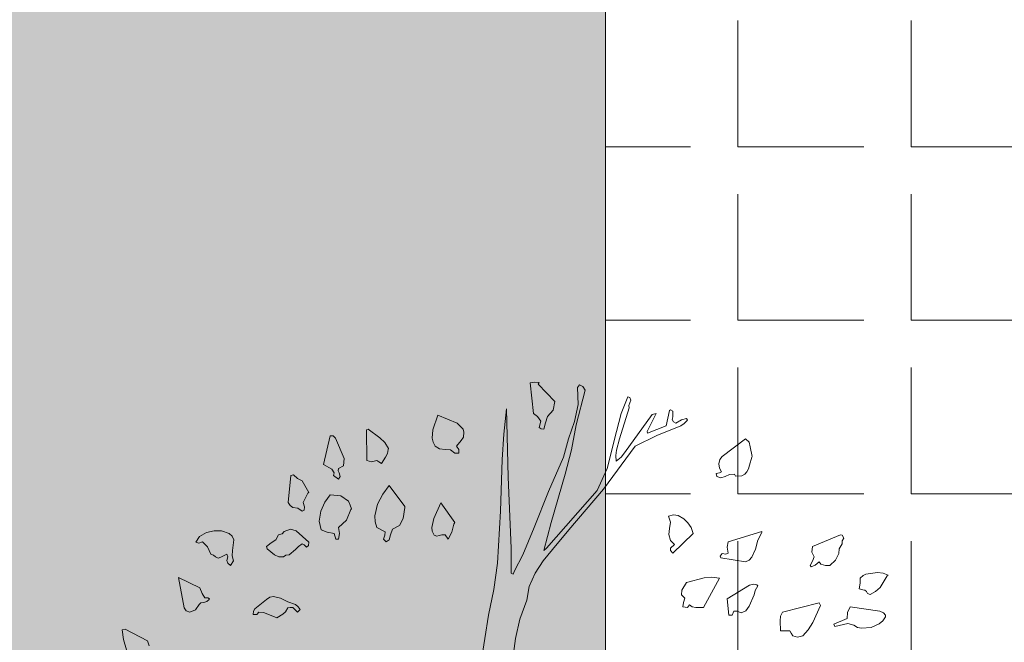
# Model space of a CAD drawing. Units: inches. Extents: x 84 to 1044, y -280 to 906.
# Tile 8 of 105: x 481 to 521, y -104 to -79. Entities that reach past the tile are written whole.
import ezdxf

# ---------------------------------------------------------------- set-up
doc = ezdxf.new("R2010")
doc.units = ezdxf.units.IN
doc.layers.add('L-HRDS', color=32, linetype='Continuous', lineweight=18)
doc.layers.add('L-PLNT', color=114, linetype='Continuous', lineweight=15)
doc.layers.add('L-HRDS-PATT', color=23, linetype='Continuous', lineweight=9, true_color=0xc2877b)
doc.layers.add('L-PLNT-PATT', color=9, linetype='Continuous', lineweight=9, true_color=0xafd9aa)

# ---------------------------------------------------------------- blocks, each defined once
blk = doc.blocks.new('A$C37E508DF')
for p, q in [((0.6329, 1.5111), (0.6367, 1.5175)), ((0.6367, 1.5175), (0.6423, 1.5201)), ((0.6423, 1.5201), (0.6453, 1.5158)), ((0.6453, 1.5158), (0.644, 1.4879)), ((0.6826, 1.493), (0.7096, 1.5209)), ((0.7083, 1.5239), (0.7152, 1.5244)), ((0.7096, 1.5209), (0.7083, 1.5239)), ((0.7152, 1.5244), (0.7225, 1.5231)), ((0.7225, 1.5231), (0.7174, 1.4729)), ((0.5583, 1.4948), (0.5596, 1.4995)), ((0.5596, 1.4995), (0.563, 1.5003)), ((0.563, 1.5003), (0.5737, 1.4733)), ((0.6475, 1.4545), (0.6329, 1.5111)), ((0.5596, 1.4905), (0.5583, 1.4948)), ((0.5613, 1.4862), (0.5596, 1.4905)), ((0.5608, 1.4823), (0.5613, 1.4862)), ((0.5767, 1.4317), (0.5608, 1.4823)), ((0.644, 1.4879), (0.6505, 1.46)), ((0.6852, 1.4785), (0.6826, 1.493)), ((0.7589, 1.3691), (0.7615, 1.481)), ((0.7615, 1.481), (0.7658, 1.4395)), ((0.4657, 1.4622), (0.4669, 1.4652)), ((0.4669, 1.4652), (0.4755, 1.463)), ((0.4897, 1.4772), (0.4935, 1.4789)), ((0.4897, 1.4678), (0.4897, 1.4772)), ((0.4905, 1.4635), (0.4897, 1.4678)), ((0.4935, 1.4789), (0.4952, 1.478)), ((0.4952, 1.478), (0.5004, 1.4532)), ((0.5313, 1.4437), (0.5167, 1.4729)), ((0.5167, 1.4729), (0.5231, 1.4716)), ((0.5231, 1.4716), (0.5686, 1.409)), ((0.5737, 1.4733), (0.5814, 1.4437)), ((0.6946, 1.4682), (0.6852, 1.4785)), ((0.6976, 1.4579), (0.6946, 1.4682)), ((0.7109, 1.4682), (0.7053, 1.4609)), ((0.7174, 1.4729), (0.7109, 1.4682)), ((0.8421, 1.4575), (0.8739, 1.4703)), ((0.8739, 1.4703), (0.882, 1.4463)), ((0.4708, 1.4566), (0.4657, 1.4622)), ((0.4764, 1.4532), (0.4708, 1.4566)), ((0.4755, 1.463), (0.4845, 1.4575)), ((0.5154, 1.4373), (0.4764, 1.4532)), ((0.4845, 1.4575), (0.4884, 1.4596)), ((0.4884, 1.4596), (0.4905, 1.4635)), ((0.5004, 1.4532), (0.5308, 1.4412)), ((0.6552, 1.4137), (0.6475, 1.4545)), ((0.6505, 1.46), (0.6603, 1.4317)), ((0.7002, 1.4476), (0.6976, 1.4579)), ((0.7083, 1.4502), (0.7049, 1.448)), ((0.7053, 1.4609), (0.7083, 1.4502)), ((0.8323, 1.4476), (0.8357, 1.451)), ((0.8357, 1.451), (0.8421, 1.4575)), ((0.551, 1.4197), (0.5154, 1.4373)), ((0.5308, 1.4412), (0.5313, 1.4437)), ((0.5814, 1.4437), (0.5969, 1.3833)), ((0.7049, 1.448), (0.7002, 1.4476)), ((0.7658, 1.4395), (0.7684, 1.3979)), ((0.831, 1.4424), (0.8323, 1.4476)), ((0.8318, 1.4343), (0.831, 1.4424)), ((0.8353, 1.4292), (0.8318, 1.4343)), ((0.8829, 1.433), (0.8816, 1.4262)), ((0.882, 1.4463), (0.8829, 1.433)), ((0.9605, 1.4257), (0.9686, 1.4334)), ((0.9686, 1.4334), (0.9875, 1.4476)), ((0.9875, 1.4476), (0.9905, 1.4467)), ((0.9905, 1.4467), (0.9896, 1.3966)), ((1.0269, 1.3996), (1.0411, 1.433)), ((1.0411, 1.433), (1.045, 1.4365)), ((1.045, 1.4365), (1.0497, 1.4369)), ((1.0497, 1.4369), (1.0604, 1.3901)), ((0.3598, 1.403), (0.3628, 1.4189)), ((0.3628, 1.4189), (0.3649, 1.4266)), ((0.3649, 1.4266), (0.3709, 1.4317)), ((0.3709, 1.4317), (0.4086, 1.403)), ((0.6029, 1.3494), (0.551, 1.4197)), ((0.5814, 1.4133), (0.5767, 1.4317)), ((0.6603, 1.4317), (0.668, 1.4021)), ((0.8434, 1.4197), (0.8353, 1.4292)), ((0.8391, 1.4141), (0.8434, 1.4197)), ((0.8781, 1.4197), (0.8709, 1.4154)), ((0.8816, 1.4262), (0.8781, 1.4197)), ((0.9545, 1.4159), (0.9605, 1.4257)), ((0.3602, 1.4021), (0.3598, 1.403)), ((0.364, 1.3888), (0.3602, 1.4021)), ((0.4086, 1.403), (0.4125, 1.3979)), ((0.5686, 1.409), (0.5741, 1.4021)), ((0.5741, 1.4021), (0.5823, 1.3953)), ((0.5827, 1.4043), (0.5814, 1.4133)), ((0.5823, 1.3953), (0.5827, 1.4043)), ((0.6655, 1.3743), (0.6552, 1.4137)), ((0.668, 1.4021), (0.6925, 1.3455)), ((0.8395, 1.4086), (0.8391, 1.4141)), ((0.846, 1.4086), (0.8395, 1.4086)), ((0.8528, 1.4137), (0.846, 1.4086)), ((0.8619, 1.4146), (0.8528, 1.4137)), ((0.8709, 1.4154), (0.8619, 1.4146)), ((0.9549, 1.4146), (0.9545, 1.4159)), ((0.9558, 1.4077), (0.9549, 1.4146)), ((0.9592, 1.4017), (0.9558, 1.4077)), ((0.966, 1.3914), (0.9592, 1.4017)), ((0.3657, 1.3828), (0.364, 1.3888)), ((0.4125, 1.3979), (0.4142, 1.391)), ((0.4142, 1.391), (0.4134, 1.3837)), ((0.7684, 1.3979), (0.771, 1.3134)), ((0.9703, 1.3944), (0.966, 1.3914)), ((0.9733, 1.3966), (0.9703, 1.3944)), ((0.9819, 1.3944), (0.9733, 1.3966)), ((0.9896, 1.3966), (0.9819, 1.3944)), ((1.0282, 1.3876), (1.0269, 1.3996)), ((1.0359, 1.3833), (1.0282, 1.3876)), ((1.0604, 1.3901), (1.0471, 1.3824)), ((0.3683, 1.3781), (0.3657, 1.3828)), ((0.3718, 1.3738), (0.3683, 1.3781)), ((0.3765, 1.3713), (0.3718, 1.3738)), ((0.3872, 1.3708), (0.3765, 1.3713)), ((0.3885, 1.3738), (0.3872, 1.3708)), ((0.3971, 1.3734), (0.3885, 1.3738)), ((0.4039, 1.3704), (0.3971, 1.3734)), ((0.4108, 1.3683), (0.4039, 1.3704)), ((0.4134, 1.3837), (0.4099, 1.3781)), ((0.4099, 1.3781), (0.4134, 1.376)), ((0.4176, 1.37), (0.4108, 1.3683)), ((0.4134, 1.376), (0.4189, 1.3751)), ((0.4189, 1.3751), (0.4176, 1.37)), ((0.5969, 1.3833), (0.6132, 1.3472)), ((0.6882, 1.2949), (0.6655, 1.3743)), ((0.7538, 1.2529), (0.7589, 1.3691)), ((1.0334, 1.37), (1.0351, 1.376)), ((1.0359, 1.3661), (1.0334, 1.37)), ((1.0351, 1.376), (1.0368, 1.3794)), ((1.0368, 1.3794), (1.0359, 1.3833)), ((1.0441, 1.3717), (1.0359, 1.3661)), ((1.0471, 1.3824), (1.0432, 1.3764)), ((1.0432, 1.3764), (1.0441, 1.3717)), ((1.1033, 1.367), (1.1097, 1.373)), ((1.1097, 1.373), (1.114, 1.3717)), ((1.114, 1.3717), (1.1183, 1.328)), ((0.9274, 1.3215), (0.9532, 1.3554)), ((0.9532, 1.3554), (0.9635, 1.3413)), ((1.0848, 1.3443), (1.0955, 1.3631)), ((1.0955, 1.3631), (1.1033, 1.367)), ((0.6595, 1.2829), (0.6029, 1.3494)), ((0.6132, 1.3472), (0.6959, 1.2529)), ((0.6925, 1.3455), (0.7161, 1.2868)), ((0.9635, 1.3413), (0.9721, 1.325)), ((1.0197, 1.3297), (1.0321, 1.3387)), ((1.0321, 1.3387), (1.0497, 1.3404)), ((1.0497, 1.3404), (1.0587, 1.3284)), ((1.0861, 1.343), (1.0848, 1.3443)), ((1.0938, 1.328), (1.0861, 1.343)), ((0.846, 1.2949), (0.8687, 1.3271)), ((0.8687, 1.3271), (0.8803, 1.3014)), ((0.9279, 1.3194), (0.9274, 1.3215)), ((0.9721, 1.325), (0.9768, 1.3061)), ((1.0149, 1.3172), (1.0171, 1.3232)), ((1.0171, 1.3232), (1.0197, 1.3297)), ((1.0587, 1.3284), (1.0651, 1.3134)), ((1.0917, 1.3207), (1.0938, 1.328)), ((1.0925, 1.3151), (1.0917, 1.3207)), ((1.1153, 1.3228), (1.111, 1.3194)), ((1.1183, 1.328), (1.1153, 1.3228)), ((0.4717, 1.3009), (0.4807, 1.3065)), ((0.4807, 1.3065), (0.4884, 1.3074)), ((0.4884, 1.3074), (0.4965, 1.3057)), ((0.4965, 1.3057), (0.4935, 1.2954)), ((0.771, 1.3134), (0.7761, 1.2285)), ((0.9305, 1.3018), (0.9279, 1.3194)), ((0.9768, 1.3061), (0.9763, 1.2962)), ((1.0162, 1.3164), (1.0149, 1.3172)), ((1.0231, 1.2988), (1.0162, 1.3164)), ((1.0651, 1.3134), (1.0677, 1.2975)), ((1.0955, 1.3138), (1.0925, 1.3151)), ((1.1028, 1.3185), (1.0955, 1.3138)), ((1.111, 1.3194), (1.1028, 1.3185)), ((0.4597, 1.2868), (0.4648, 1.2945)), ((0.4648, 1.2945), (0.4717, 1.3009)), ((0.4935, 1.2954), (0.4948, 1.2855)), ((0.7002, 1.2495), (0.6882, 1.2949)), ((0.8473, 1.2924), (0.846, 1.2949)), ((0.8507, 1.2795), (0.8473, 1.2924)), ((0.8803, 1.3014), (0.8833, 1.2872)), ((0.9365, 1.2902), (0.9305, 1.3018)), ((0.9476, 1.2842), (0.9365, 1.2902)), ((0.9763, 1.2962), (0.9733, 1.2868)), ((1.0359, 1.2868), (1.0231, 1.2988)), ((1.0677, 1.2975), (1.0647, 1.2829)), ((0.2101, 1.2696), (0.2127, 1.2744)), ((0.2127, 1.2744), (0.2152, 1.2752)), ((0.2152, 1.2752), (0.2611, 1.2559)), ((0.3439, 1.2804), (0.3992, 1.2636)), ((0.3439, 1.2787), (0.3439, 1.2804)), ((0.3507, 1.2662), (0.3439, 1.2787)), ((0.4562, 1.2774), (0.4597, 1.2868)), ((0.4897, 1.2452), (0.4562, 1.2774)), ((0.4961, 1.2756), (0.4935, 1.2658)), ((0.4948, 1.2855), (0.4961, 1.2756)), ((0.6865, 1.2508), (0.6595, 1.2829)), ((0.7161, 1.2868), (0.7349, 1.2422)), ((0.8567, 1.2679), (0.8507, 1.2795)), ((0.8619, 1.2752), (0.8567, 1.2679)), ((0.867, 1.2752), (0.8619, 1.2752)), ((0.8713, 1.2739), (0.867, 1.2752)), ((0.8756, 1.2726), (0.8713, 1.2739)), ((0.8799, 1.2744), (0.8756, 1.2726)), ((0.8829, 1.2808), (0.8799, 1.2744)), ((0.8833, 1.2872), (0.8829, 1.2808)), ((0.951, 1.2748), (0.9476, 1.2842)), ((0.9532, 1.2666), (0.951, 1.2748)), ((0.9733, 1.2868), (0.9596, 1.2799)), ((0.9596, 1.2799), (0.9605, 1.2744)), ((0.9605, 1.2744), (0.9626, 1.2679)), ((1.0347, 1.2769), (1.0359, 1.2868)), ((1.0359, 1.2679), (1.0347, 1.2769)), ((1.0432, 1.2774), (1.0402, 1.2679)), ((1.0544, 1.2791), (1.0432, 1.2774)), ((1.0647, 1.2829), (1.0544, 1.2791)), ((1.0848, 1.2628), (1.1054, 1.2817)), ((1.1054, 1.2817), (1.1148, 1.2842)), ((1.1148, 1.2842), (1.1247, 1.2804)), ((1.1247, 1.2804), (1.1281, 1.2765)), ((1.1281, 1.2765), (1.1341, 1.2752)), ((1.1341, 1.2752), (1.1384, 1.2666)), ((1.2075, 1.2666), (1.21, 1.2726)), ((1.21, 1.2726), (1.2147, 1.2774)), ((1.2147, 1.2774), (1.2276, 1.2817)), ((1.2276, 1.2817), (1.2392, 1.2817)), ((1.2392, 1.2817), (1.2521, 1.2787)), ((1.2521, 1.2787), (1.2632, 1.2722)), ((1.2632, 1.2722), (1.2692, 1.2628)), ((0.2127, 1.2654), (0.2101, 1.2696)), ((0.2127, 1.2602), (0.2127, 1.2654)), ((0.2174, 1.2521), (0.2127, 1.2602)), ((0.2611, 1.2559), (0.262, 1.2465)), ((0.3546, 1.2516), (0.3507, 1.2662)), ((0.3992, 1.2636), (0.4005, 1.2546)), ((0.4935, 1.2658), (0.4867, 1.2589)), ((0.4867, 1.2589), (0.4935, 1.2529)), ((0.9583, 1.2636), (0.9532, 1.2666)), ((0.9626, 1.2679), (0.9583, 1.2636)), ((1.0402, 1.2679), (1.0359, 1.2679)), ((1.0852, 1.2576), (1.0848, 1.2628)), ((1.0883, 1.2546), (1.0852, 1.2576)), ((1.0921, 1.2585), (1.0883, 1.2546)), ((1.0955, 1.2602), (1.0921, 1.2585)), ((1.1015, 1.2559), (1.0955, 1.2602)), ((1.1063, 1.2508), (1.1015, 1.2559)), ((1.1384, 1.2666), (1.1461, 1.2619)), ((1.1461, 1.2619), (1.1539, 1.2559)), ((1.1539, 1.2559), (1.1526, 1.2521)), ((1.2096, 1.2491), (1.2075, 1.2666)), ((1.2585, 1.2636), (1.2503, 1.2551)), ((1.2645, 1.2615), (1.2585, 1.2636)), ((1.2692, 1.2628), (1.2645, 1.2615)), ((0.2182, 1.2443), (0.2174, 1.2521)), ((0.2234, 1.2336), (0.2182, 1.2443)), ((0.262, 1.2465), (0.2586, 1.2388)), ((0.3602, 1.2383), (0.3546, 1.2516)), ((0.4005, 1.2546), (0.3992, 1.2452)), ((0.3992, 1.2452), (0.4026, 1.2431)), ((0.4026, 1.2431), (0.4086, 1.2443)), ((0.4086, 1.2443), (0.4121, 1.2401)), ((0.4121, 1.2401), (0.4112, 1.2375)), ((0.4931, 1.2491), (0.4897, 1.2452)), ((0.4935, 1.2529), (0.4931, 1.2491)), ((0.7015, 1.2323), (0.6865, 1.2508)), ((0.6959, 1.2529), (0.7002, 1.2495)), ((0.7349, 1.2422), (0.7482, 1.216)), ((0.7538, 1.2122), (0.7538, 1.2529)), ((1.117, 1.2422), (1.1063, 1.2508)), ((1.1221, 1.2418), (1.117, 1.2422)), ((1.126, 1.2388), (1.1221, 1.2418)), ((1.141, 1.2422), (1.1337, 1.2388)), ((1.1526, 1.2521), (1.141, 1.2422)), ((1.2079, 1.2323), (1.21, 1.2409)), ((1.21, 1.2409), (1.2096, 1.2491)), ((1.2186, 1.2431), (1.2173, 1.2392)), ((1.2285, 1.2383), (1.2186, 1.2431)), ((1.2405, 1.2418), (1.2371, 1.2388)), ((1.2448, 1.2431), (1.2405, 1.2418)), ((1.2503, 1.2551), (1.2448, 1.2431)), ((0.2328, 1.2251), (0.2234, 1.2336)), ((0.2401, 1.2251), (0.2328, 1.2251)), ((0.2474, 1.2268), (0.2401, 1.2251)), ((0.2504, 1.2306), (0.2474, 1.2268)), ((0.2568, 1.2255), (0.2504, 1.2306)), ((0.2633, 1.2229), (0.2568, 1.2255)), ((0.2586, 1.2388), (0.2611, 1.2319)), ((0.2611, 1.2319), (0.265, 1.2251)), ((0.265, 1.2251), (0.2633, 1.2229)), ((0.3649, 1.2336), (0.3602, 1.2383)), ((0.3709, 1.2306), (0.3649, 1.2336)), ((0.4112, 1.2375), (0.3709, 1.2306)), ((0.7148, 1.2126), (0.7015, 1.2323)), ((0.7761, 1.2285), (0.7821, 1.1856)), ((1.1337, 1.2388), (1.126, 1.2388)), ((1.2126, 1.2251), (1.2079, 1.2323)), ((1.2169, 1.2285), (1.2126, 1.2251)), ((1.2186, 1.2332), (1.2169, 1.2285)), ((1.2173, 1.2392), (1.2186, 1.2332)), ((1.2328, 1.2366), (1.2285, 1.2383)), ((1.2371, 1.2388), (1.2328, 1.2366)), ((0.1376, 1.2092), (0.1458, 1.2126)), ((0.1389, 1.2079), (0.1376, 1.2092)), ((0.1505, 1.189), (0.1389, 1.2079)), ((0.1458, 1.2126), (0.1548, 1.2135)), ((0.1548, 1.2135), (0.1741, 1.2109)), ((0.1741, 1.2109), (0.1784, 1.2083)), ((0.1784, 1.2083), (0.1831, 1.204)), ((0.7246, 1.1908), (0.7148, 1.2126)), ((0.7482, 1.216), (0.7508, 1.2109)), ((0.7508, 1.2109), (0.7538, 1.2122)), ((0.1831, 1.204), (0.1831, 1.1959)), ((0.1831, 1.1959), (0.1848, 1.1865)), ((0.3507, 1.1916), (0.352, 1.1933)), ((0.355, 1.1839), (0.3507, 1.1916)), ((0.352, 1.1933), (0.3576, 1.1942)), ((0.3576, 1.1942), (0.364, 1.1929)), ((0.364, 1.1929), (0.4005, 1.1702)), ((0.4134, 1.204), (0.4258, 1.2058)), ((0.4391, 1.156), (0.4134, 1.204)), ((0.4258, 1.2058), (0.4382, 1.2045)), ((0.4382, 1.2045), (0.4669, 1.1972)), ((0.4669, 1.1972), (0.4747, 1.1843)), ((1.2628, 1.1882), (1.2975, 1.2053)), ((1.2975, 1.2053), (1.2885, 1.1556)), ((0.1582, 1.1822), (0.1505, 1.189)), ((0.1668, 1.1775), (0.1582, 1.1822)), ((0.1711, 1.1792), (0.1668, 1.1775)), ((0.1728, 1.1826), (0.1711, 1.1792)), ((0.1758, 1.1847), (0.1728, 1.1826)), ((0.1788, 1.1852), (0.1758, 1.1847)), ((0.1848, 1.1865), (0.1788, 1.1852)), ((0.3563, 1.177), (0.355, 1.1839)), ((0.3645, 1.1586), (0.3563, 1.177)), ((0.4751, 1.177), (0.47, 1.1714)), ((0.4747, 1.1843), (0.4751, 1.177)), ((0.7281, 1.168), (0.7246, 1.1908)), ((0.7821, 1.1856), (0.7911, 1.1436)), ((1.2546, 1.1719), (1.2589, 1.1792)), ((1.2589, 1.1792), (1.2628, 1.1882)), ((0.2478, 1.1594), (0.2504, 1.1637)), ((0.2607, 1.1316), (0.2478, 1.1594)), ((0.2504, 1.1637), (0.3104, 1.1487)), ((0.4005, 1.1702), (0.3979, 1.1436)), ((0.4622, 1.1607), (0.458, 1.1573)), ((0.4657, 1.156), (0.4622, 1.1607)), ((0.47, 1.1714), (0.4721, 1.1646)), ((0.4721, 1.1646), (0.473, 1.1573)), ((0.7396, 1.1371), (0.7281, 1.168)), ((1.102, 1.1573), (1.1063, 1.1612)), ((1.1063, 1.1612), (1.1187, 1.1655)), ((1.1187, 1.1655), (1.1307, 1.1714)), ((1.1307, 1.1714), (1.1423, 1.1744)), ((1.1423, 1.1744), (1.1483, 1.1732)), ((1.1483, 1.1732), (1.1539, 1.1693)), ((1.1539, 1.1693), (1.1727, 1.1543)), ((1.2469, 1.1702), (1.2495, 1.1723)), ((1.2478, 1.1693), (1.2469, 1.1702)), ((1.2516, 1.1659), (1.2478, 1.1693)), ((1.2495, 1.1723), (1.2546, 1.1719)), ((1.2563, 1.1646), (1.2516, 1.1659)), ((1.2611, 1.1637), (1.2563, 1.1646)), ((1.2641, 1.1612), (1.2611, 1.1637)), ((1.2701, 1.1522), (1.2641, 1.1612)), ((0.1419, 1.1436), (0.1449, 1.1474)), ((0.1419, 1.141), (0.1419, 1.1436)), ((0.1449, 1.1474), (0.1509, 1.1504)), ((0.1509, 1.1504), (0.1994, 1.1573)), ((0.1994, 1.1573), (0.2041, 1.1479)), ((0.2041, 1.1479), (0.2045, 1.138)), ((0.3104, 1.1487), (0.3134, 1.1423)), ((0.37, 1.1509), (0.3645, 1.1586)), ((0.3778, 1.1474), (0.37, 1.1509)), ((0.3842, 1.15), (0.3778, 1.1474)), ((0.3898, 1.15), (0.3842, 1.15)), ((0.3923, 1.1436), (0.3898, 1.15)), ((0.3979, 1.1436), (0.3923, 1.1436)), ((0.4519, 1.1564), (0.4391, 1.156)), ((0.458, 1.1573), (0.4519, 1.1564)), ((0.473, 1.1573), (0.4657, 1.156)), ((0.7911, 1.1436), (0.8027, 1.0677)), ((1.099, 1.153), (1.102, 1.1573)), ((1.1033, 1.1487), (1.099, 1.153)), ((1.111, 1.156), (1.1033, 1.1487)), ((1.1153, 1.1564), (1.111, 1.156)), ((1.1191, 1.1556), (1.1153, 1.1564)), ((1.1226, 1.1492), (1.1191, 1.1556)), ((1.1273, 1.1453), (1.1226, 1.1492)), ((1.1367, 1.1393), (1.1273, 1.1453)), ((1.1517, 1.1453), (1.1367, 1.1393)), ((1.1586, 1.1483), (1.1517, 1.1453)), ((1.1663, 1.1487), (1.1586, 1.1483)), ((1.1697, 1.1449), (1.1663, 1.1487)), ((1.1757, 1.1449), (1.1697, 1.1449)), ((1.1727, 1.1543), (1.1749, 1.1504)), ((1.1749, 1.1504), (1.1757, 1.1449)), ((1.2791, 1.1487), (1.2701, 1.1522)), ((1.2851, 1.1509), (1.2791, 1.1487)), ((1.2885, 1.1556), (1.2851, 1.1509)), ((0.1462, 1.1342), (0.1419, 1.141)), ((0.1522, 1.1294), (0.1462, 1.1342)), ((0.1655, 1.1234), (0.1522, 1.1294)), ((0.1938, 1.1273), (0.1878, 1.1234)), ((0.2032, 1.1303), (0.1938, 1.1273)), ((0.2247, 1.1251), (0.2032, 1.1303)), ((0.2045, 1.138), (0.226, 1.129)), ((0.226, 1.129), (0.2247, 1.1251)), ((0.268, 1.1196), (0.2607, 1.1316)), ((0.3134, 1.1423), (0.3139, 1.1346)), ((0.3139, 1.1346), (0.3134, 1.1183)), ((0.7469, 1.1054), (0.7396, 1.1371)), ((0.181, 1.1226), (0.1655, 1.1234)), ((0.1878, 1.1234), (0.181, 1.1226)), ((0.277, 1.1101), (0.268, 1.1196)), ((0.2959, 1.1144), (0.2933, 1.1101)), ((0.2984, 1.1179), (0.2959, 1.1144)), ((0.3066, 1.1179), (0.2984, 1.1179)), ((0.3134, 1.1183), (0.3066, 1.1179)), ((1.3485, 1.102), (1.385, 1.1209)), ((1.385, 1.1209), (1.3897, 1.1196)), ((1.3897, 1.1196), (1.3875, 1.1037)), ((0.2856, 1.108), (0.277, 1.1101)), ((0.2933, 1.1101), (0.2856, 1.108)), ((0.7512, 1.0728), (0.7469, 1.1054)), ((1.3455, 1.0934), (1.3485, 1.102)), ((1.3875, 1.1037), (1.3828, 1.087))]:
    blk.add_line(p, q)

msp = doc.modelspace()

# ---------------------------------------------------------------- hatches: boundary and pattern name
at = {"layer": 'L-HRDS-PATT', "transparency": 33554567}
h = msp.add_hatch(dxfattribs=at)
h.set_pattern_fill('ANGLE', color=256)
h.set_pattern_definition([(0, (0, 0), (0, 6.985), [5.08, -1.905]), (90, (0, 0), (-6.985, 4e-16), [5.08, -1.905])])
h.paths.add_polyline_path([(650.074, 31.12), (504.574, 31.12), (504.574, -112.88), (504.574, -121.88), (624.574, -121.88), (624.574, -112.88), (650.074, -112.88)])
at = {"layer": 'L-PLNT-PATT', "transparency": 33554597}
h = msp.add_hatch(color=256, dxfattribs=at)
h.dxf.hatch_style = 1
h.paths.add_polyline_path([(504.574, -40.88), (455.074, -40.88), (455.074, -112.88), (504.574, -112.88)])

# ---------------------------------------------------------------- linework, layer by layer
at = {"layer": 'L-HRDS'}
msp.add_line((504.574, -112.88), (504.574, 31.12), dxfattribs=at)

# ---------------------------------------------------------------- block references
at = {"layer": 'L-PLNT', "xscale": -24.64361536662419, "yscale": 24.64361536662419, "zscale": 24.64361536662419}
msp.add_blockref('A$C37E508DF', (519.355, -130.86), dxfattribs=at)

doc.saveas('drawing.dxf')
